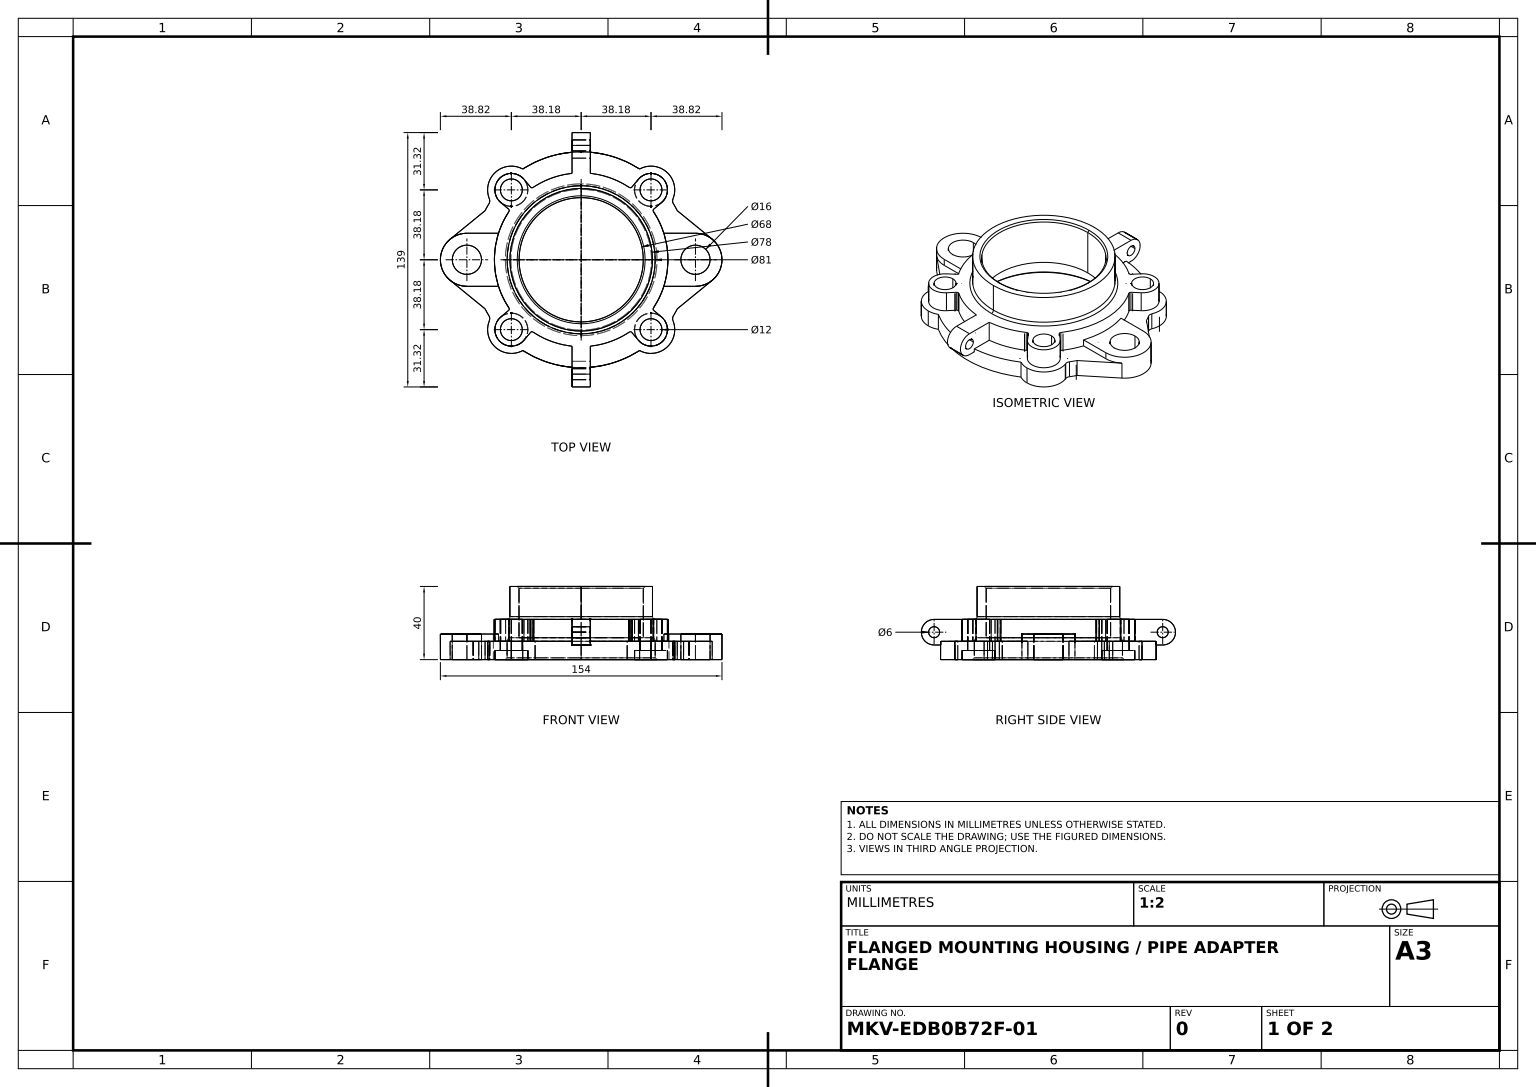
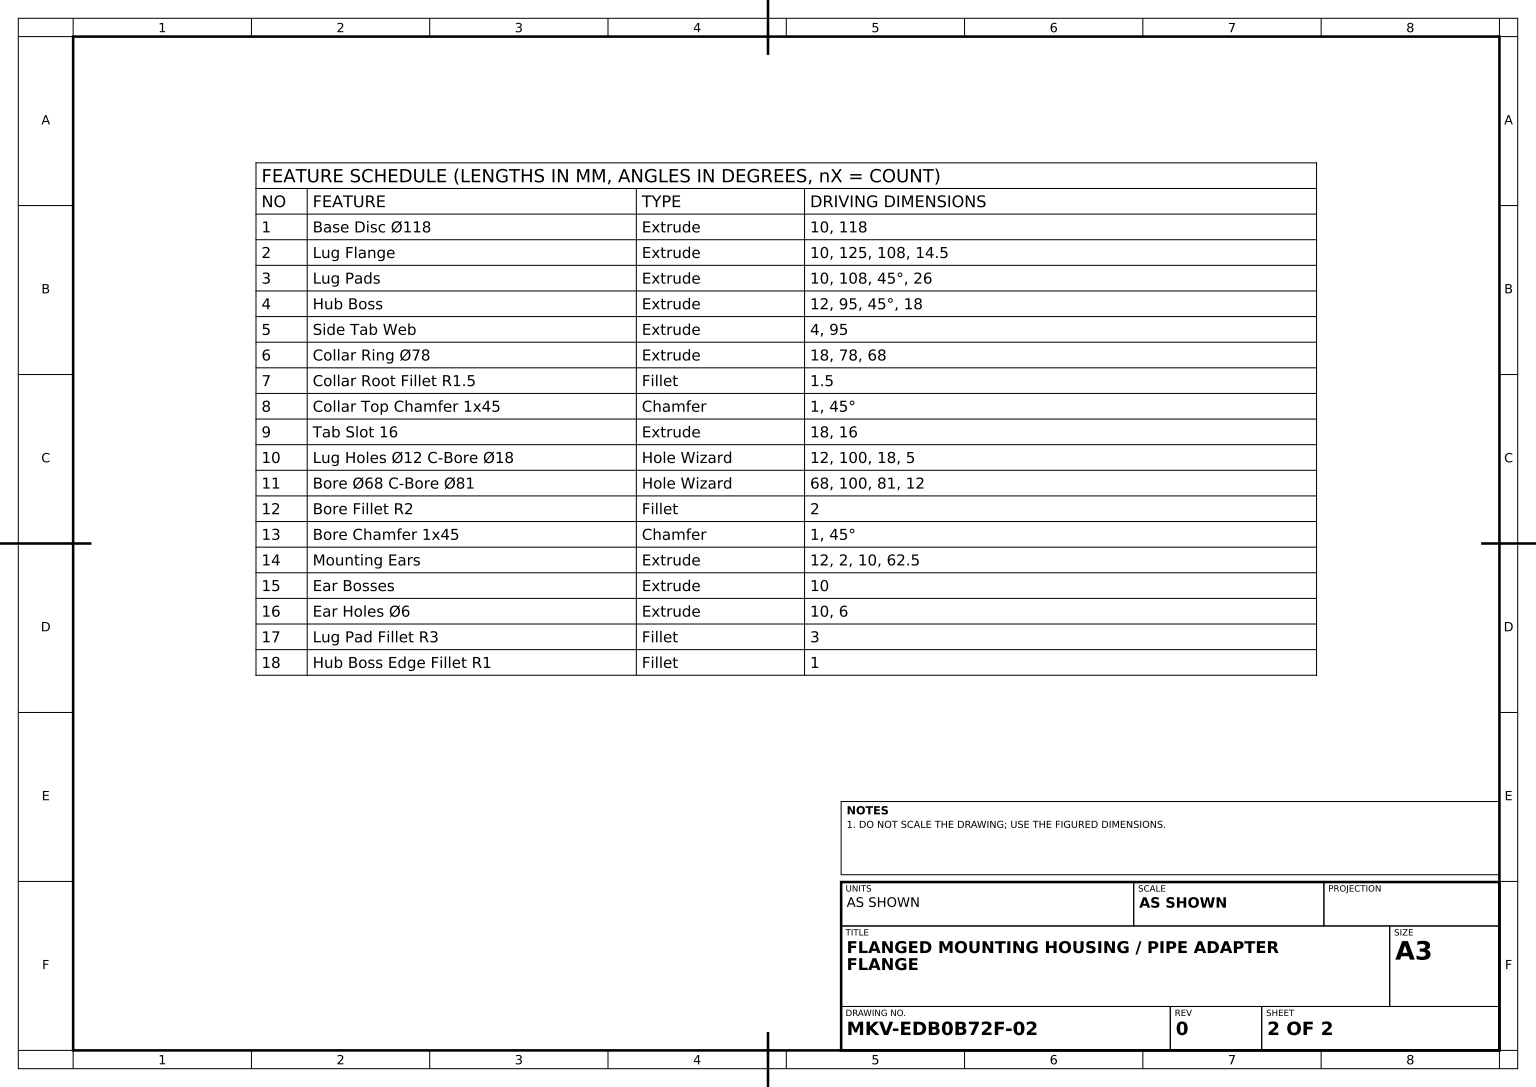
from build123d import *

# Parameters (mm, degrees)
BASE_DISC_SKETCH_R                 = 59
BASE_DISC_118_DEPTH                = 10
LUG_FLANGE_DEPTH                   = 10
LUG_START                          = -10
LUG_PADS_DEPTH                     = 10
HUB_BOSS_DEPTH                     = 12
SIDE_TAB_WEB_DEPTH                 = 4
COLLAR_RING_SKETCH_R               = 39
COLLAR_RING_SKETCH_R_2             = 34
COLLAR_RING_78_DEPTH               = 18
COLLAR_ROOT_FILLET_R1_5_R          = 1.5
COLLAR_TOP_CHAMFER_1X45_SIZE       = 1
TAB_SLOT_SKETCH_R                  = 8
TAB_SLOT_16_DEPTH                  = 18
LUG_HOLES_12_C_BORE_18_D           = 12
LUG_HOLES_12_C_BORE_18_DEPTH       = 99.95498987
LUG_HOLES_12_C_BORE_18_CBORE_D     = 18
LUG_HOLES_12_C_BORE_18_CBORE_DEPTH = 5
BORE_68_C_BORE_81_D                = 68
BORE_68_C_BORE_81_DEPTH            = 99.788526395
BORE_68_C_BORE_81_CBORE_D          = 81
BORE_68_C_BORE_81_CBORE_DEPTH      = 12
BORE_FILLET_R2_R                   = 2
BORE_CHAMFER_1X45_SIZE             = 1
MOUNTING_EARS_DEPTH                = 12
MOUNTING_EARS_DEPTH_BACK           = 2
MOUNTING_EAR_SKETCH_W              = 10
MOUNTING_EAR_SKETCH_H              = 15.263890931
EAR_BOSS_SKETCH_R                  = 7
EAR_BOSSES_DEPTH                   = 10
EAR_HOLE_SKETCH_R                  = 3
EAR_HOLES_6_DEPTH                  = 10
LUG_PAD_FILLET_R3_R                = 3
HUB_BOSS_EDGE_FILLET_R1_R          = 1


with BuildPart() as part:
    # Base Disc Sketch → Base Disc Ø118 (new body)
    with BuildSketch(Plane(origin=(0, 0, 0), x_dir=(1, 0, 0), z_dir=(0, 1, 0))):
        with Locations(Location((0, 0, 0), (0, 0, 270))):
            Circle(BASE_DISC_SKETCH_R)
    extrude(amount=BASE_DISC_118_DEPTH)

    # Lug Flange Sketch → Lug Flange (add)
    with BuildSketch(Plane.XZ):
        with BuildLine():
            Line((71.664, 11.237041604), (52.548788257, 26.825824363))
            ThreePointArc((52.548788257, 26.825824363), (0, 59), (-52.548788257, 26.825824363))
            Line((-52.548788257, 26.825824363), (-71.664, 11.237041604))
            ThreePointArc((-71.664, 11.237041604), (-77, 0), (-71.664, -11.237041604))
            Line((-71.664, -11.237041604), (-52.548788257, -26.825824363))
            ThreePointArc((-52.548788257, -26.825824363), (0, -59), (52.548788257, -26.825824363))
            Line((52.548788257, -26.825824363), (71.664, -11.237041604))
            ThreePointArc((71.664, -11.237041604), (77, 0), (71.664, 11.237041604))
        make_face()
    extrude(amount=-LUG_FLANGE_DEPTH)

    # Lug Pads Sketch → Lug Pads (add)
    with BuildSketch(Plane(origin=(0, 10, 0), x_dir=(1, 0, 0), z_dir=(0, 1, 0)).offset(LUG_START)):
        with BuildLine():
            ThreePointArc((-49.595662085, -31.957320012), (-47.376154339, -47.376154339), (-31.957320012, -49.595662085))
            ThreePointArc((-31.957320012, -49.595662085), (0, -59), (31.957320012, -49.595662085))
            ThreePointArc((31.957320012, -49.595662085), (47.376154339, -47.376154339), (49.595662085, -31.957320012))
            ThreePointArc((49.595662085, -31.957320012), (59, 0), (49.595662085, 31.957320012))
            ThreePointArc((49.595662085, 31.957320012), (47.376154339, 47.376154339), (31.957320012, 49.595662085))
            ThreePointArc((31.957320012, 49.595662085), (0, 59), (-31.957320012, 49.595662085))
            ThreePointArc((-31.957320012, 49.595662085), (-47.376154339, 47.376154339), (-49.595662085, 31.957320012))
            ThreePointArc((-49.595662085, 31.957320012), (-59, 0), (-49.595662085, -31.957320012))
        make_face()
    extrude(amount=LUG_PADS_DEPTH)

    # Hub Boss Sketch → Hub Boss (add)
    with BuildSketch(Plane(origin=(0, 10, 0), x_dir=(1, 0, 0), z_dir=(0, 1, 0))):
        with BuildLine():
            Line((-31.311610651, -43.995261545), (-27.097752399, -39.012329012))
            ThreePointArc((-27.097752399, -39.012329012), (0, -47.5), (27.097752399, -39.012329012))
            Line((27.097752399, -39.012329012), (31.311610651, -43.995261545))
            ThreePointArc((31.311610651, -43.995261545), (44.547727215, -44.547727215), (43.995261545, -31.311610651))
            Line((43.995261545, -31.311610651), (39.012329012, -27.097752399))
            ThreePointArc((39.012329012, -27.097752399), (47.5, 0), (39.012329012, 27.097752399))
            Line((39.012329012, 27.097752399), (43.995261545, 31.311610651))
            ThreePointArc((43.995261545, 31.311610651), (44.547727215, 44.547727215), (31.311610651, 43.995261545))
            Line((31.311610651, 43.995261545), (27.097752399, 39.012329012))
            ThreePointArc((27.097752399, 39.012329012), (0, 47.5), (-27.097752399, 39.012329012))
            Line((-27.097752399, 39.012329012), (-31.311610651, 43.995261545))
            ThreePointArc((-31.311610651, 43.995261545), (-44.547727215, 44.547727215), (-43.995261545, 31.311610651))
            Line((-43.995261545, 31.311610651), (-39.012329012, 27.097752399))
            ThreePointArc((-39.012329012, 27.097752399), (-47.5, 0), (-39.012329012, -27.097752399))
            Line((-39.012329012, -27.097752399), (-43.995261545, -31.311610651))
            ThreePointArc((-43.995261545, -31.311610651), (-44.547727215, -44.547727215), (-31.311610651, -43.995261545))
        make_face()
    extrude(amount=HUB_BOSS_DEPTH)

    # Side Tab Sketch → Side Tab Web (add)
    with BuildSketch(Plane(origin=(0, 10, 0), x_dir=(1, 0, 0), z_dir=(0, 1, 0))):
        with BuildLine():
            Line((-62.5, 14.5), (-45.232731512, 14.5))
            ThreePointArc((-45.232731512, 14.5), (0, 47.5), (45.232731512, 14.5))
            Line((45.232731512, 14.5), (62.5, 14.5))
            ThreePointArc((62.5, 14.5), (77, 0), (62.5, -14.5))
            Line((62.5, -14.5), (45.232731512, -14.5))
            ThreePointArc((45.232731512, -14.5), (0, -47.5), (-45.232731512, -14.5))
            Line((-45.232731512, -14.5), (-62.5, -14.5))
            ThreePointArc((-62.5, -14.5), (-77, 0), (-62.5, 14.5))
        make_face()
    extrude(amount=SIDE_TAB_WEB_DEPTH)

    # Collar Ring Sketch → Collar Ring Ø78 (add)
    with BuildSketch(Plane(origin=(0, 22, 0), x_dir=(1, 0, 0), z_dir=(0, 1, 0))):
        with Locations(Location((0, 0, 0), (0, 0, 90))):
            Circle(COLLAR_RING_SKETCH_R)
        with Locations(Location((0, 0, 0), (0, 0, 270))):
            Circle(COLLAR_RING_SKETCH_R_2, mode=Mode.SUBTRACT)
    extrude(amount=COLLAR_RING_78_DEPTH)

    # Collar Root Fillet R1.5
    collar_root_fillet_r1_5_edges = [part.edges().sort_by_distance(p)[0] for p in [
        (0, 22, 39),
    ]]
    fillet(collar_root_fillet_r1_5_edges, radius=COLLAR_ROOT_FILLET_R1_5_R)

    # Collar Top Chamfer 1x45
    collar_top_chamfer_1x45_edges = [part.edges().sort_by_distance(p)[0] for p in [
        (0, 40, -34),
    ]]
    chamfer(collar_top_chamfer_1x45_edges, length=COLLAR_TOP_CHAMFER_1X45_SIZE)

    # Tab Slot Sketch → Tab Slot 16 (cut)
    with BuildSketch(Plane(origin=(0, 14, 0), x_dir=(1, 0, 0), z_dir=(0, 1, 0))):
        with Locations(Location((-62.5, 0, 0), (0, 0, 270))):
            Circle(TAB_SLOT_SKETCH_R)
        with Locations(Location((62.5, 0, 0), (0, 0, 270))):
            Circle(TAB_SLOT_SKETCH_R)
    extrude(amount=-TAB_SLOT_16_DEPTH, mode=Mode.SUBTRACT)

    # Lug Holes Ø12 C-Bore Ø18
    with Locations(Plane(origin=(-38.183766184, 0, 38.183766184), x_dir=(0, 0, -1), z_dir=(0, -1, 0))):
        with Locations((0, 0), (0, 76.367532368), (76.367532368, 76.367532368), (76.367532368, 0)):
            CounterBoreHole(LUG_HOLES_12_C_BORE_18_D / 2, LUG_HOLES_12_C_BORE_18_CBORE_D / 2, LUG_HOLES_12_C_BORE_18_CBORE_DEPTH, depth=LUG_HOLES_12_C_BORE_18_DEPTH)

    # Bore Ø68 C-Bore Ø81
    with Locations(Plane(origin=(0, 0, 0), x_dir=(0, 0, -1), z_dir=(0, -1, 0))):
        with Locations((0, 0)):
            CounterBoreHole(BORE_68_C_BORE_81_D / 2, BORE_68_C_BORE_81_CBORE_D / 2, BORE_68_C_BORE_81_CBORE_DEPTH, depth=BORE_68_C_BORE_81_DEPTH)

    # Bore Fillet R2
    bore_fillet_r2_edges = [part.edges().sort_by_distance(p)[0] for p in [
        (0, 12, 40.5),
    ]]
    fillet(bore_fillet_r2_edges, radius=BORE_FILLET_R2_R)

    # Bore Chamfer 1x45
    bore_chamfer_1x45_edges = [part.edges().sort_by_distance(p)[0] for p in [
        (0, 0, 40.5),
    ]]
    chamfer(bore_chamfer_1x45_edges, length=BORE_CHAMFER_1X45_SIZE)

    # Mounting Ear Sketch → Mounting Ears (add, two sides: drawn at the far end of the back side and taken through both)
    with BuildSketch(Plane(origin=(0, 10, 0), x_dir=(1, 0, 0), z_dir=(0, 1, 0)).offset(-MOUNTING_EARS_DEPTH_BACK)):
        with Locations((0, 54.868054535)):
            Rectangle(MOUNTING_EAR_SKETCH_W, MOUNTING_EAR_SKETCH_H)
        with Locations((0, -54.868054535)):
            Rectangle(MOUNTING_EAR_SKETCH_W, MOUNTING_EAR_SKETCH_H)
    extrude(amount=MOUNTING_EARS_DEPTH + MOUNTING_EARS_DEPTH_BACK)

    # Ear Boss Sketch → Ear Bosses (add)
    with BuildSketch(Plane(origin=(5, 0, 0), x_dir=(0, 0, -1), z_dir=(1, 0, 0))):
        with Locations((62.5, 15)):
            Circle(EAR_BOSS_SKETCH_R)
        with Locations((-62.5, 15)):
            Circle(EAR_BOSS_SKETCH_R)
    extrude(amount=-EAR_BOSSES_DEPTH)

    # Ear Hole Sketch → Ear Holes Ø6 (cut)
    with BuildSketch(Plane(origin=(5, 0, 0), x_dir=(0, 0, -1), z_dir=(1, 0, 0))):
        with Locations((-62.5, 15)):
            Circle(EAR_HOLE_SKETCH_R)
        with Locations((62.5, 15)):
            Circle(EAR_HOLE_SKETCH_R)
    extrude(amount=-EAR_HOLES_6_DEPTH, mode=Mode.SUBTRACT)

    # Lug Pad Fillet R3
    lug_pad_fillet_r3_edges = [part.edges().sort_by_distance(p)[0] for p in [
        (-49.595662085, 5, 31.957320012),
        (49.595662085, 5, -31.957320012),
        (-49.595662085, 5, -31.957320012),
        (49.595662085, 5, 31.957320012),
    ]]
    fillet(lug_pad_fillet_r3_edges, radius=LUG_PAD_FILLET_R3_R)

    # Hub Boss Edge Fillet R1
    hub_boss_edge_fillet_r1_edges = [part.edges().sort_by_distance(p)[0] for p in [
        (-27.097752399, 16, 39.012329012),
        (27.097752399, 16, 39.012329012),
        (39.012329012, 16, 27.097752399),
        (39.012329012, 16, -27.097752399),
        (27.097752399, 16, -39.012329012),
        (-27.097752399, 16, -39.012329012),
        (-39.012329012, 16, -27.097752399),
        (-39.012329012, 16, 27.097752399),
    ]]
    fillet(hub_boss_edge_fillet_r1_edges, radius=HUB_BOSS_EDGE_FILLET_R1_R)


solid = part.part
